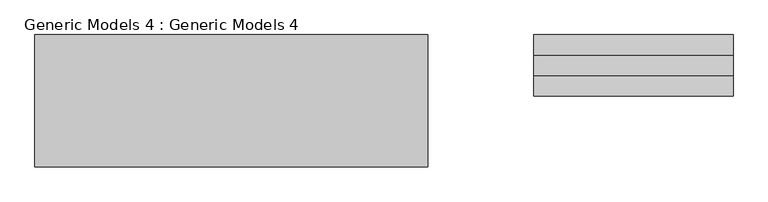
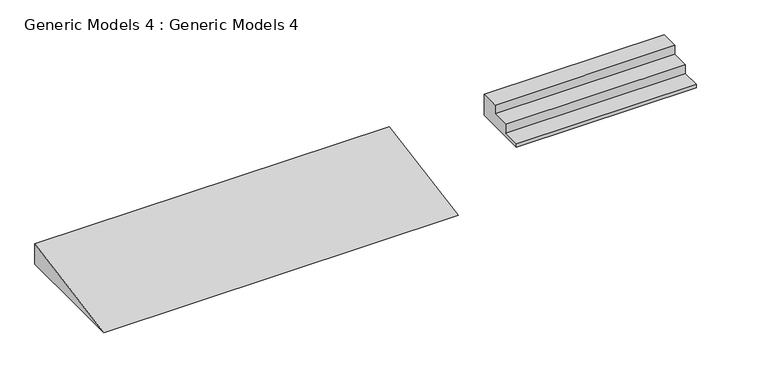
"""IFC4 building model written with IfcOpenShell, lengths in millimetres: proxy geometry, Generic Models 4 : Generic Models 4."""

from ifc_helpers import new_model, si_unit, frame, origin, place, context, project, spatial, polyline, outline, extrude, source, transform, mapped, element, save


def generic_models_4_generic_models_4_16c068d2(model_context):
    return source(origin(), model_context, "Body", "SweptSolid", [
        extrude(outline(polyline([(-3493.1367893, 0.0), (-3239.1367893, 0.0), (-3239.1367893, -304.8), (-4001.1367893, -304.8), (-4001.1367893, -254.0), (-3747.1367893, -254.0), (-3747.1367893, -127.0), (-3493.1367893, -127.0), (-3493.1367893, 0.0)])), frame((-3291.6025595, 0.0, 0.0), z_axis=(1.0, 0.0, 0.0), x_axis=(0.0, 1.0, 0.0)), (0.0, 0.0, 1.0), 2475.0),
        extrude(outline(polyline([(-4204.3367893, -304.8), (-4883.7867893, -304.8), (-3239.1367893, -10.2358209), (-3239.1367893, -304.8), (-4204.3367893, -304.8)])), frame((-9480.9025595, 0.0, 0.0), z_axis=(1.0, 0.0, 0.0), x_axis=(0.0, 1.0, 0.0)), (0.0, 0.0, 1.0), 4876.8),
    ])


if __name__ == "__main__":
    model = new_model("IFC4")
    model_context = context("Model", 3, world=origin())
    ifc_project = project(units=[si_unit("LENGTHUNIT", "METRE", prefix="MILLI")], contexts=[model_context])
    site = spatial("IfcSite", under=ifc_project)
    building = spatial("IfcBuilding", under=site)
    placement = place(None, origin())
    generic_models_4_generic_models_4_shape = generic_models_4_generic_models_4_16c068d2(model_context)
    element("IfcBuildingElementProxy", 1, Name="Generic Models 4 : Generic Models 4", ObjectType="Generic Models 4 : Generic Models 4", at=placement, inside=building, context=model_context, shape_type="MappedRepresentation", body=[
        mapped(generic_models_4_generic_models_4_shape, transform((0.0, 0.0, 0.0), x_axis=(1.0, 0.0, 0.0), y_axis=(0.0, 1.0, 0.0), z_axis=(0.0, 0.0, 1.0))),
    ])
    save(model, "model.ifc")
